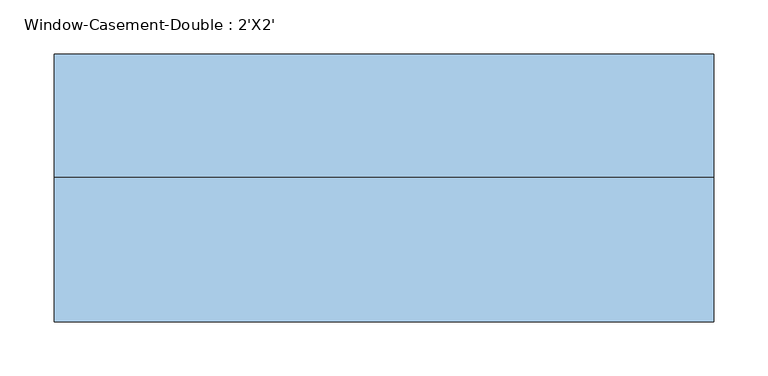
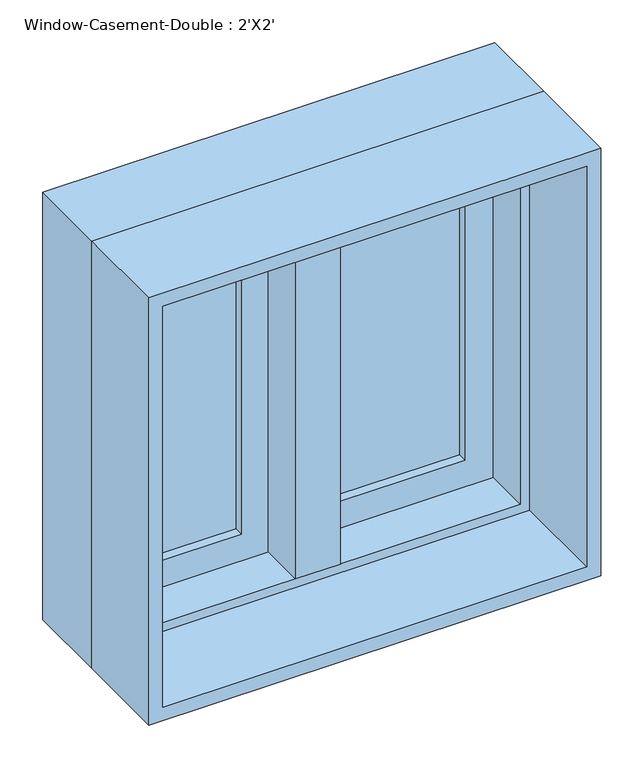
"""IFC4 building model written with IfcOpenShell, lengths in millimetres: window geometry, Window-Casement-Double : 2'X2'."""

from ifc_helpers import new_model, si_unit, frame, origin, place, context, project, spatial, polyline, outline, extrude, faceted_brep, source, transform, mapped, element, save


def window_casement_double_2_x2_3fc3773f(model_context):
    return source(origin(), model_context, "Body", "SolidModel", [
        faceted_brep([(9.525, 133.35, 1511.3), (-9.525, 133.35, 1511.3), (-9.525, 82.55, 1511.3), (9.525, 82.55, 1511.3), (9.525, 133.35, 927.1), (9.525, 82.55, 927.1), (-9.525, 82.55, 927.1), (-9.525, 133.35, 927.1), (-9.525, 82.55, 946.15), (-9.525, 82.55, 1492.25), (-30.1625, 82.55, 946.15), (-30.1625, 82.55, 1492.25), (-30.1625, 19.05, 946.15), (-30.1625, 19.05, 1492.25), (30.1625, 19.05, 946.15), (30.1625, 19.05, 1492.25), (30.1625, 82.55, 946.15), (30.1625, 82.55, 1492.25), (9.525, 82.55, 946.15), (9.525, 82.55, 1492.25)], [[[0, 1, 2, 3]], [[4, 5, 6, 7]], [[1, 0, 4, 7]], [[2, 1, 7, 6, 8, 9]], [[9, 8, 10, 11]], [[11, 10, 12, 13]], [[13, 12, 14, 15]], [[15, 14, 16, 17]], [[17, 16, 18, 19]], [[0, 3, 19, 18, 5, 4]], [[18, 8, 6, 5]], [[9, 19, 3, 2]], [[8, 18, 16, 14, 12, 10]], [[19, 9, 11, 13, 15, 17]]]),
        extrude(outline(polyline([(-66.675, 114.3), (-66.675, 107.95), (-234.95, 107.95), (-234.95, 114.3), (-66.675, 114.3)])), frame((0.0, 0.0, 984.25), z_axis=(0.0, 0.0, 1.0), x_axis=(1.0, 0.0, 0.0)), (0.0, 0.0, 1.0), 469.9),
        extrude(outline(polyline([(-234.95, 95.25), (-234.95, 101.6), (-66.675, 101.6), (-66.675, 95.25), (-234.95, 95.25)])), frame((0.0, 0.0, 984.25), z_axis=(0.0, 0.0, 1.0), x_axis=(1.0, 0.0, 0.0)), (0.0, 0.0, 1.0), 469.9),
        extrude(outline(polyline([(234.95, 114.3), (234.95, 107.95), (66.675, 107.95), (66.675, 114.3), (234.95, 114.3)])), frame((0.0, 0.0, 984.25), z_axis=(0.0, 0.0, 1.0), x_axis=(1.0, 0.0, 0.0)), (0.0, 0.0, 1.0), 469.9),
        extrude(outline(polyline([(66.675, 95.25), (66.675, 101.6), (234.95, 101.6), (234.95, 95.25), (66.675, 95.25)])), frame((0.0, 0.0, 984.25), z_axis=(0.0, 0.0, 1.0), x_axis=(1.0, 0.0, 0.0)), (0.0, 0.0, 1.0), 469.9),
        extrude(outline(polyline([(1511.3, -292.1), (927.1, -292.1), (927.1, -9.525), (1511.3, -9.525), (1511.3, -292.1)]), holes=[polyline([(1454.15, -66.675), (984.25, -66.675), (984.25, -234.95), (1454.15, -234.95), (1454.15, -66.675)])]), frame((0.0, 82.55, 0.0), z_axis=(0.0, 1.0, 0.0), x_axis=(0.0, 0.0, 1.0)), (0.0, 0.0, 1.0), 44.45),
        extrude(outline(polyline([(927.1, 292.1), (1511.3, 292.1), (1511.3, 9.525), (927.1, 9.525), (927.1, 292.1)]), holes=[polyline([(984.25, 66.675), (1454.15, 66.675), (1454.15, 234.95), (984.25, 234.95), (984.25, 66.675)])]), frame((0.0, 82.55, 0.0), z_axis=(0.0, 1.0, 0.0), x_axis=(0.0, 0.0, 1.0)), (0.0, 0.0, 1.0), 44.45),
        extrude(outline(polyline([(1524.0, -304.8), (914.4, -304.8), (914.4, 304.8), (1524.0, 304.8), (1524.0, -304.8)]), holes=[polyline([(1504.95, 285.75), (933.45, 285.75), (933.45, -285.75), (1504.95, -285.75), (1504.95, 285.75)])]), frame((0.0, -114.3, 0.0), z_axis=(0.0, 1.0, 0.0), x_axis=(0.0, 0.0, 1.0)), (0.0, 0.0, 1.0), 133.35),
        faceted_brep([(273.05, 82.55, 1492.25), (273.05, 19.05, 1492.25), (-273.05, 19.05, 1492.25), (-273.05, 82.55, 1492.25), (292.1, 133.35, 1511.3), (292.1, 82.55, 1511.3), (-292.1, 82.55, 1511.3), (-292.1, 133.35, 1511.3), (304.8, 19.05, 1524.0), (304.8, 133.35, 1524.0), (-304.8, 133.35, 1524.0), (-304.8, 19.05, 1524.0), (-273.05, 19.05, 946.15), (-273.05, 82.55, 946.15), (-292.1, 82.55, 927.1), (-292.1, 133.35, 927.1), (-304.8, 133.35, 914.4), (-304.8, 19.05, 914.4), (273.05, 19.05, 946.15), (273.05, 82.55, 946.15), (292.1, 82.55, 927.1), (292.1, 133.35, 927.1), (304.8, 133.35, 914.4), (304.8, 19.05, 914.4)], [[[0, 1, 2, 3]], [[4, 5, 6, 7]], [[8, 9, 10, 11]], [[3, 2, 12, 13]], [[7, 6, 14, 15]], [[11, 10, 16, 17]], [[13, 12, 18, 19]], [[15, 14, 20, 21]], [[17, 16, 22, 23]], [[11, 17, 23, 8], [1, 18, 12, 2]], [[19, 18, 1, 0]], [[5, 20, 14, 6], [3, 13, 19, 0]], [[21, 20, 5, 4]], [[23, 22, 9, 8]], [[9, 22, 16, 10], [7, 15, 21, 4]]]),
    ])


if __name__ == "__main__":
    model = new_model("IFC4")
    model_context = context("Model", 3, world=origin())
    ifc_project = project(units=[si_unit("LENGTHUNIT", "METRE", prefix="MILLI")], contexts=[model_context])
    site = spatial("IfcSite", under=ifc_project)
    building = spatial("IfcBuilding", under=site)
    placement = place(None, origin())
    window_casement_double_2_x2_shape = window_casement_double_2_x2_3fc3773f(model_context)
    element("IfcWindow", 1, ObjectType="Window-Casement-Double : 2'X2'", at=placement, inside=building, context=model_context, shape_type="MappedRepresentation", body=[
        mapped(window_casement_double_2_x2_shape, transform((0.0, 0.0, 0.0), x_axis=(1.0, 0.0, 0.0), y_axis=(0.0, 1.0, 0.0), z_axis=(0.0, 0.0, 1.0))),
    ])
    save(model, "model.ifc")

# Revit data of these elements
# Type "Window-Casement-Double : 2'X2'"
#   Type Mark = "20"
#   Fire Rating = "0.5h"
#   Assembly Code = "B2020100"
#   Analytic Construction = "Double glazing - domestic"
#   Frame Extension [instance default] = 0' - 0 1/4"
#   Window Inset [instance default] = 0' - 0"
#   Wall Thickness [instance default] = 0' - 6"
#   Interior Wall Closure [instance default] = 0' - 2 1/4"
#   Half Width = 1' - 0"
#   Visual Light Transmittance = 0.81
#   Thermal Resistance (R) = 1.8146 (h·ft²·°F)/BTU
#   Solar Heat Gain Coefficient = 0.76
#   Rough Width = 2' - 0 1/2"
#   Rough Height = 2' - 0 1/2"
#   Height = 2' - 0"
#   Heat Transfer Coefficient (U) = 0.5511 BTU/(h·ft²·°F)
#   Exterior Wall Closure [instance default] = 0' - 1 1/4"
#   Extension Jamb [instance default] = 0' - 2 1/4"
#   Default Sill Height = 3' - 0"
#   Width = 2' - 0"
#   Muntin Visibility = yes
#   Interior Trim Visibility [instance default] = yes
#   Exterior Trim Visibility [instance default] = yes
#   Extension Jamb Visibility [instance default] = yes
#   Interior Trim Material = Wood - Stained
#   Muntin Pattern = Muntin Pattern_2x2 : Muntin Pattern_2x2
#   Interior Trim = Trim-Window-Interior-Flat : Picture Frame
#   Interior Frame Material = Wood - Stained
#   Glass Panel Material = Glass
#   Exterior Trim Material = Clad - White
#   Exterior Trim = Trim-Window-Exterior-Flat : with Sill
#   Exterior Frame Material = Clad - White
#   Wall Closure = (empty or 0)
# Element 1 (IfcWindow, "Window-Casement-Double : 2'X2'")
#   Wall Thickness = 0' - 9"
#   Extension Jamb = 0' - 5 1/4"
#   Materials on its faces: "Wood - Stained", "Glass", "Clad - White"
# Materials
#   "Wood - Stained": class "Wood", colour RGB 224 178 126, transparency 0, Cost = 0
#   "Glass": class "Glass", colour RGB 0 128 192, transparency 0.75, Description = "Soda Lime Glass", Cost = 0
#   "Clad - White": class "Wood", colour RGB 242 242 238, transparency 0, Cost = 0
